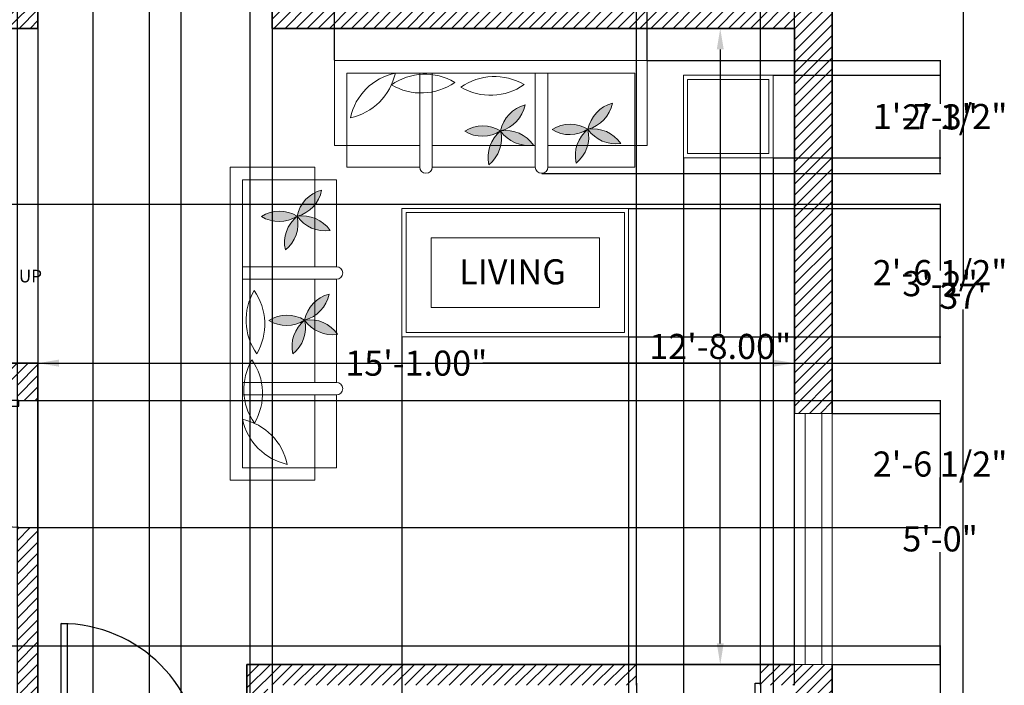
# Model space of a CAD drawing. Units: inches. Extents: x -302 to 383, y -29 to 550.
# Tile 3 of 4: x 147 to 383, y 149 to 308. Entities that reach past the tile are written whole.
import ezdxf

# ---------------------------------------------------------------- set-up
doc = ezdxf.new("R2010")
doc.units = ezdxf.units.IN
doc.header["$MEASUREMENT"] = 0
for name, color, linetype, lineweight in [('A-ANNO-DIMS', 3, 'Continuous', 18), ('A-ANNO-TEXT', 7, 'Continuous', 18), ('A-AREA-IDEN', 2, 'Continuous', 25), ('A-DOOR', 4, 'Continuous', 25), ('A-FURN', 1, 'Continuous', 18), ('A-FURN-PATT', 2, 'Continuous', 13), ('A-GLAZ', 2, 'Continuous', 18), ('A-WALL', 7, 'Continuous', 35), ('A-WALL-PATT', 252, 'Continuous', 13)]:
    doc.layers.add(name, color=color, linetype=linetype, lineweight=lineweight)
doc.styles.get("Standard").update_dxf_attribs({"font": 'arial.ttf'})
doc.dimstyles.get("Standard").update_dxf_attribs({"dimtxt": 6, "dimasz": 0.18, "dimexe": 0.18, "dimexo": 0.0625, "dimgap": 0.09, "dimtad": 0, "dimtih": 1, "dimtoh": 1, "dimzin": 0, "dimdsep": 46, "dimlunit": 3, "dimtxsty": 'Standard', "dimcen": 0.09, "dimadec": 0, "dimazin": 0, "dimtfac": 1, "dimtofl": 0, "dimtmove": 0, "dimatfit": 3, "dimfxl": 1, "dimtolj": 1, "dimtzin": 0, "dimarcsym": 0})

# ---------------------------------------------------------------- blocks, each defined once
blk = doc.blocks.new('*U2')
for p, q in [((0, 0), (0, -6)), ((40, 0), (40, -6))]:
    blk.add_line(p, q)
blk.add_lwpolyline([(0, 0), (0, 40), (1.75, 40), (1.75, 0)], close=True)
blk.add_arc((0, 0), 40, 0, 90)
blk = doc.blocks.new('*D13')
at = {"layer": 'A-ANNO-DIMS', "color": 0, "lineweight": -2, "transparency": 16777216}
for p, q in [((151.7, 226.34), (151.7, 226.45)), ((156.7, 226.27), (226.26, 226.27)), ((327.7, 226.27), (258.14, 226.27)), ((332.7, 226.34), (332.7, 226.45))]:
    blk.add_line(p, q, dxfattribs=at)
at = {"layer": 'A-ANNO-DIMS', "color": 0, "transparency": 16777216}
for points in [[(156.7, 227.11), (156.7, 225.44), (151.7, 226.27)], [(327.7, 227.11), (327.7, 225.44), (332.7, 226.27)]]:
    blk.add_solid(points, dxfattribs=at)
at = {"layer": 'Defpoints', "color": 0, "transparency": 16777216}
for p in [(151.7, 226.27), (332.7, 226.27), (332.7, 226.27)]:
    blk.add_point(p, dxfattribs=at)
at = {"layer": 'A-ANNO-DIMS', "color": 0, "transparency": 16777216, "insert": (242.2, 226.27), "char_height": 6, "attachment_point": 5}
blk.add_mtext('\\A1;15\'-1.00"', dxfattribs=at)
blk = doc.blocks.new('*D14')
at = {"layer": 'A-ANNO-DIMS', "color": 0, "lineweight": -2, "transparency": 16777216}
for p, q in [((332.63, 306.27), (314.73, 306.27)), ((314.91, 301.27), (314.91, 233.43)), ((314.91, 159.27), (314.91, 227.12)), ((332.63, 154.27), (314.73, 154.27))]:
    blk.add_line(p, q, dxfattribs=at)
at = {"layer": 'A-ANNO-DIMS', "color": 0, "transparency": 16777216}
for points in [[(314.08, 301.27), (315.74, 301.27), (314.91, 306.27)], [(314.08, 159.27), (315.74, 159.27), (314.91, 154.27)]]:
    blk.add_solid(points, dxfattribs=at)
at = {"layer": 'Defpoints', "color": 0, "transparency": 16777216}
for p in [(332.7, 306.27), (314.91, 154.27), (332.7, 154.27)]:
    blk.add_point(p, dxfattribs=at)
at = {"layer": 'A-ANNO-DIMS', "color": 0, "transparency": 16777216, "insert": (314.91, 230.27), "char_height": 6, "attachment_point": 5}
blk.add_mtext('\\A1;12\'-8.00"', dxfattribs=at)
blk = doc.blocks.new('*D22')
at = {"layer": 'A-ANNO-DIMS', "color": 0, "lineweight": -2, "transparency": 16777216}
for p, q in [((341.76, 464.27), (373.16, 464.27)), ((372.98, 459.27), (372.98, 245.43)), ((372.98, 25.27), (372.98, 239.12)), ((341.76, 20.27), (373.16, 20.27))]:
    blk.add_line(p, q, dxfattribs=at)
at = {"layer": 'A-ANNO-DIMS', "color": 0, "transparency": 16777216}
for points in [[(372.15, 459.27), (373.82, 459.27), (372.98, 464.27)], [(372.15, 25.27), (373.82, 25.27), (372.98, 20.27)]]:
    blk.add_solid(points, dxfattribs=at)
at = {"layer": 'Defpoints', "color": 0, "transparency": 16777216}
for p in [(341.7, 464.27), (341.7, 20.27), (372.98, 20.27)]:
    blk.add_point(p, dxfattribs=at)
at = {"layer": 'A-ANNO-DIMS', "color": 0, "transparency": 16777216, "insert": (372.98, 242.27), "char_height": 6, "attachment_point": 5}
blk.add_mtext("\\A1;37'", dxfattribs=at)
blk = doc.blocks.new('SOFA-LEAF-TRIO')
for points in [[(0, 0, 0.294318), (10.77, 10.69, 0.294318)], [(9.82, 7.86, 0.294318), (24.97, 8.46, 0.294318)], [(26.41, 7.31, 0.294318), (41.57, 7.92, 0.294318)]]:
    blk.add_lwpolyline(points, format="xyb", close=True)
blk = doc.blocks.new('SOFA-FLORAL-MOTIF-A')
h = blk.add_hatch(color=256)
h.dxf.hatch_style = 1
h.paths.add_polyline_path([(0, 8, 0.287656), (8.55, 8.07, 0.287656)])
h.paths.add_polyline_path([(14.4, 14.32, 0.287656), (8.55, 8.07, 0.287656)])
h.paths.add_polyline_path([(8.55, 8.07, 0.287656), (5.73, 0, 0.287656)])
h.paths.add_polyline_path([(8.55, 8.07, 0.287656), (16.41, 4.69, 0.287656)])
for centre, start, end in [((16.45, 6.53), 104.7854, 168.9781), ((6.5, 15.85), 284.7854, 348.9781), ((4.34, 1.22), 58.4247, 122.6174), ((4.21, 14.85), 238.4247, 302.6174), ((13.58, 1.79), 128.6278, 192.8205), ((0.7, 6.29), 308.6278, 12.8205), ((9.78, 0.12), 34.5823, 98.775), ((15.18, 12.64), 214.5823, 278.775)]:
    blk.add_arc(centre, 8.05, start, end)
blk = doc.blocks.new('SOFA-FLORAL-MOTIF-B')
h = blk.add_hatch(color=256)
h.dxf.hatch_style = 1
h.paths.add_polyline_path([(0, 8, 0.287656), (8.55, 8.07, 0.287656)])
h.paths.add_polyline_path([(14.4, 14.32, 0.287656), (8.55, 8.07, 0.287656)])
h.paths.add_polyline_path([(5.73, 0, 0.287656), (8.55, 8.07, 0.287656)])
h.paths.add_polyline_path([(16.41, 4.69, 0.287656), (8.55, 8.07, 0.287656)])
for centre, start, end in [((16.45, 6.53), 104.7854, 168.9781), ((6.5, 15.85), 284.7854, 348.9781), ((4.34, 1.22), 58.4247, 122.6174), ((4.21, 14.85), 238.4247, 302.6174), ((13.58, 1.79), 128.6278, 192.8205), ((0.7, 6.29), 308.6278, 12.8205), ((9.78, 0.12), 34.5823, 98.775), ((15.18, 12.64), 214.5823, 278.775)]:
    blk.add_arc(centre, 8.05, start, end)
blk = doc.blocks.new('*D33')
at = {"layer": 'A-ANNO-DIMS', "color": 0, "lineweight": -2, "transparency": 16777216}
for p, q in [((210.8, 127.61), (210.8, 125.91)), ((221.35, 127.61), (221.35, 125.91)), ((210.98, 126.09), (221.17, 126.09)), ((221.35, 126.09), (221.53, 126.09))]:
    blk.add_line(p, q, dxfattribs=at)
at = {"layer": 'A-ANNO-DIMS', "color": 0, "transparency": 16777216}
for points in [[(210.98, 126.12), (210.98, 126.06), (210.8, 126.09)], [(221.17, 126.12), (221.17, 126.06), (221.35, 126.09)]]:
    blk.add_solid(points, dxfattribs=at)
at = {"layer": 'Defpoints', "color": 0, "transparency": 16777216}
for p in [(210.8, 127.68), (221.35, 127.68), (221.35, 126.09)]:
    blk.add_point(p, dxfattribs=at)
at = {"layer": 'A-ANNO-DIMS', "color": 0, "transparency": 16777216, "insert": (276.32, 126.09), "char_height": 6, "attachment_point": 5}
blk.add_mtext('\\A1;TABLE LAMP 0\'-10 1/2" TYP.', dxfattribs=at)
blk = doc.blocks.new('*D45')
at = {"layer": 'A-ANNO-DIMS', "color": 0, "lineweight": -2, "transparency": 16777216}
for p, q in [((341.76, 214.27), (367.68, 214.27)), ((367.5, 214.09), (367.5, 187.43)), ((367.5, 154.45), (367.5, 181.12)), ((341.76, 154.27), (367.68, 154.27))]:
    blk.add_line(p, q, dxfattribs=at)
at = {"layer": 'A-ANNO-DIMS', "color": 0, "transparency": 16777216}
for points in [[(367.47, 214.09), (367.53, 214.09), (367.5, 214.27)], [(367.47, 154.45), (367.53, 154.45), (367.5, 154.27)]]:
    blk.add_solid(points, dxfattribs=at)
at = {"layer": 'Defpoints', "color": 0, "transparency": 16777216}
for p in [(341.7, 214.27), (367.5, 214.27), (341.7, 154.27)]:
    blk.add_point(p, dxfattribs=at)
at = {"layer": 'A-ANNO-DIMS', "color": 0, "transparency": 16777216, "insert": (367.5, 184.27), "char_height": 6, "attachment_point": 5}
blk.add_mtext('\\A1;5\'-0"', dxfattribs=at)
blk = doc.blocks.new('*D50')
at = {"layer": 'A-ANNO-DIMS', "color": 0, "lineweight": -2, "transparency": 16777216}
for p, q in [((178.34, 359.21), (178.34, -5.71)), ((202.4, 359.21), (202.4, -5.71)), ((178.52, -5.53), (182.25, -5.53)), ((202.22, -5.53), (198.48, -5.53))]:
    blk.add_line(p, q, dxfattribs=at)
at = {"layer": 'A-ANNO-DIMS', "color": 0, "transparency": 16777216}
for points in [[(178.52, -5.5), (178.52, -5.56), (178.34, -5.53)], [(202.22, -5.5), (202.22, -5.56), (202.4, -5.53)]]:
    blk.add_solid(points, dxfattribs=at)
at = {"layer": 'Defpoints', "color": 0, "transparency": 16777216}
for p in [(178.34, 359.27), (202.4, 359.27), (202.4, -5.53)]:
    blk.add_point(p, dxfattribs=at)
at = {"layer": 'A-ANNO-DIMS', "color": 0, "transparency": 16777216, "insert": (190.37, -5.53), "char_height": 6, "attachment_point": 5}
blk.add_mtext('\\A1;2\'-0"', dxfattribs=at)
blk = doc.blocks.new('*D51')
at = {"layer": 'A-ANNO-DIMS', "color": 0, "lineweight": -2, "transparency": 16777216}
for p, q in [((146.76, 217.32), (367.68, 217.32)), ((367.5, 217.14), (367.5, 205.35)), ((367.5, 187.18), (367.5, 198.97)), ((146.76, 187), (367.68, 187))]:
    blk.add_line(p, q, dxfattribs=at)
at = {"layer": 'A-ANNO-DIMS', "color": 0, "transparency": 16777216}
for points in [[(367.47, 217.14), (367.53, 217.14), (367.5, 217.32)], [(367.47, 187.18), (367.53, 187.18), (367.5, 187)]]:
    blk.add_solid(points, dxfattribs=at)
at = {"layer": 'Defpoints', "color": 0, "transparency": 16777216}
for p in [(146.7, 217.32), (367.5, 217.32), (146.7, 187)]:
    blk.add_point(p, dxfattribs=at)
at = {"layer": 'A-ANNO-DIMS', "color": 0, "transparency": 16777216, "insert": (367.5, 202.16), "char_height": 6, "attachment_point": 5}
blk.add_mtext('\\A1;2\'-6 1/2"', dxfattribs=at)
blk = doc.blocks.new('*D53')
at = {"layer": 'A-ANNO-DIMS', "color": 0, "lineweight": -2, "transparency": 16777216}
for p, q in [((294.85, 149.34), (294.85, 541.25)), ((295.03, 541.07), (324.38, 541.07)), ((324.56, 149.34), (324.56, 541.25)), ((324.56, 541.07), (324.74, 541.07))]:
    blk.add_line(p, q, dxfattribs=at)
at = {"layer": 'A-ANNO-DIMS', "color": 0, "transparency": 16777216}
for points in [[(295.03, 541.1), (295.03, 541.04), (294.85, 541.07)], [(324.38, 541.1), (324.38, 541.04), (324.56, 541.07)]]:
    blk.add_solid(points, dxfattribs=at)
at = {"layer": 'Defpoints', "color": 0, "transparency": 16777216}
for p in [(324.56, 541.07), (294.85, 149.27), (324.56, 149.27)]:
    blk.add_point(p, dxfattribs=at)
at = {"layer": 'A-ANNO-DIMS', "color": 0, "transparency": 16777216, "insert": (339.85, 541.07), "char_height": 6, "attachment_point": 5}
blk.add_mtext('\\A1;2\'-5 1/2"', dxfattribs=at)
blk = doc.blocks.new('*D56')
at = {"layer": 'A-ANNO-DIMS', "color": 0, "lineweight": -2, "transparency": 16777216}
for p, q in [((134.76, 264.27), (367.68, 264.27)), ((367.5, 264.09), (367.5, 248.43)), ((367.5, 226.45), (367.5, 242.12)), ((134.76, 226.27), (367.68, 226.27))]:
    blk.add_line(p, q, dxfattribs=at)
at = {"layer": 'A-ANNO-DIMS', "color": 0, "transparency": 16777216}
for points in [[(367.47, 264.09), (367.53, 264.09), (367.5, 264.27)], [(367.47, 226.45), (367.53, 226.45), (367.5, 226.27)]]:
    blk.add_solid(points, dxfattribs=at)
at = {"layer": 'Defpoints', "color": 0, "transparency": 16777216}
for p in [(134.7, 264.27), (367.5, 264.27), (134.7, 226.27)]:
    blk.add_point(p, dxfattribs=at)
at = {"layer": 'A-ANNO-DIMS', "color": 0, "transparency": 16777216, "insert": (367.5, 245.27), "char_height": 6, "attachment_point": 5}
blk.add_mtext('\\A1;3\'-2"', dxfattribs=at)
blk = doc.blocks.new('*D58')
at = {"layer": 'A-ANNO-DIMS', "color": 0, "lineweight": -2, "transparency": 16777216}
for p, q in [((50.76, 158.73), (367.68, 158.73)), ((367.5, 158.55), (367.5, 109.19)), ((367.5, 53.45), (367.5, 102.81)), ((50.76, 53.27), (367.68, 53.27))]:
    blk.add_line(p, q, dxfattribs=at)
at = {"layer": 'A-ANNO-DIMS', "color": 0, "transparency": 16777216}
for points in [[(367.47, 158.55), (367.53, 158.55), (367.5, 158.73)], [(367.47, 53.45), (367.53, 53.45), (367.5, 53.27)]]:
    blk.add_solid(points, dxfattribs=at)
at = {"layer": 'Defpoints', "color": 0, "transparency": 16777216}
for p in [(50.7, 158.73), (367.5, 158.73), (50.7, 53.27)]:
    blk.add_point(p, dxfattribs=at)
at = {"layer": 'A-ANNO-DIMS', "color": 0, "transparency": 16777216, "insert": (367.5, 106), "char_height": 6, "attachment_point": 5}
blk.add_mtext('\\A1;8\'-9 1/2"', dxfattribs=at)
blk = doc.blocks.new('*D60')
at = {"layer": 'A-ANNO-DIMS', "color": 0, "lineweight": -2, "transparency": 16777216}
for p, q in [((164.84, 447.21), (164.84, -5.71)), ((185.84, 447.21), (185.84, -5.71)), ((165.02, -5.53), (167.56, -5.53)), ((185.66, -5.53), (183.12, -5.53))]:
    blk.add_line(p, q, dxfattribs=at)
at = {"layer": 'A-ANNO-DIMS', "color": 0, "transparency": 16777216}
for points in [[(165.02, -5.5), (165.02, -5.56), (164.84, -5.53)], [(185.66, -5.5), (185.66, -5.56), (185.84, -5.53)]]:
    blk.add_solid(points, dxfattribs=at)
at = {"layer": 'Defpoints', "color": 0, "transparency": 16777216}
for p in [(164.84, 447.27), (185.84, 447.27), (185.84, -5.53)]:
    blk.add_point(p, dxfattribs=at)
at = {"layer": 'A-ANNO-DIMS', "color": 0, "transparency": 16777216, "insert": (175.34, -5.53), "char_height": 6, "attachment_point": 5}
blk.add_mtext('\\A1;1\'-9"', dxfattribs=at)
blk = doc.blocks.new('*D62')
at = {"layer": 'A-ANNO-DIMS', "color": 0, "lineweight": -2, "transparency": 16777216}
for p, q in [((222.62, 298.67), (222.62, 541.25)), ((222.8, 541.07), (251.95, 541.07)), ((297.27, 541.07), (268.11, 541.07)), ((297.45, 298.67), (297.45, 541.25))]:
    blk.add_line(p, q, dxfattribs=at)
at = {"layer": 'A-ANNO-DIMS', "color": 0, "transparency": 16777216}
for points in [[(222.8, 541.1), (222.8, 541.04), (222.62, 541.07)], [(297.27, 541.1), (297.27, 541.04), (297.45, 541.07)]]:
    blk.add_solid(points, dxfattribs=at)
at = {"layer": 'Defpoints', "color": 0, "transparency": 16777216}
for p in [(297.45, 541.07), (222.62, 298.61), (297.45, 298.61)]:
    blk.add_point(p, dxfattribs=at)
at = {"layer": 'A-ANNO-DIMS', "color": 0, "transparency": 16777216, "insert": (260.03, 541.07), "char_height": 6, "attachment_point": 5}
blk.add_mtext('\\A1;6\'-3"', dxfattribs=at)
blk = doc.blocks.new('*D63')
at = {"layer": 'A-ANNO-DIMS', "color": 0, "lineweight": -2, "transparency": 16777216}
for p, q in [((297.51, 298.61), (367.68, 298.61)), ((367.5, 298.43), (367.5, 288.28)), ((367.5, 271.82), (367.5, 281.97)), ((272.23, 271.64), (367.68, 271.64))]:
    blk.add_line(p, q, dxfattribs=at)
at = {"layer": 'A-ANNO-DIMS', "color": 0, "transparency": 16777216}
for points in [[(367.47, 298.43), (367.53, 298.43), (367.5, 298.61)], [(367.47, 271.82), (367.53, 271.82), (367.5, 271.64)]]:
    blk.add_solid(points, dxfattribs=at)
at = {"layer": 'Defpoints', "color": 0, "transparency": 16777216}
for p in [(297.45, 298.61), (272.17, 271.64), (367.5, 271.64)]:
    blk.add_point(p, dxfattribs=at)
at = {"layer": 'A-ANNO-DIMS', "color": 0, "transparency": 16777216, "insert": (367.5, 285.13), "char_height": 6, "attachment_point": 5}
blk.add_mtext('\\A1;2\'-3"', dxfattribs=at)
blk = doc.blocks.new('*D64')
at = {"layer": 'A-ANNO-DIMS', "color": 0, "lineweight": -2, "transparency": 16777216}
for p, q in [((238.76, 232.51), (238.76, -5.71)), ((292.99, 232.51), (292.99, -5.71)), ((238.94, -5.53), (257.69, -5.53)), ((292.81, -5.53), (274.06, -5.53))]:
    blk.add_line(p, q, dxfattribs=at)
at = {"layer": 'A-ANNO-DIMS', "color": 0, "transparency": 16777216}
for points in [[(238.94, -5.5), (238.94, -5.56), (238.76, -5.53)], [(292.81, -5.5), (292.81, -5.56), (292.99, -5.53)]]:
    blk.add_solid(points, dxfattribs=at)
at = {"layer": 'Defpoints', "color": 0, "transparency": 16777216}
for p in [(238.76, 232.57), (292.99, 232.57), (292.99, -5.53)]:
    blk.add_point(p, dxfattribs=at)
at = {"layer": 'A-ANNO-DIMS', "color": 0, "transparency": 16777216, "insert": (265.88, -5.53), "char_height": 6, "attachment_point": 5}
blk.add_mtext('\\A1;4\'-6"', dxfattribs=at)
blk = doc.blocks.new('*D65')
at = {"layer": 'A-ANNO-DIMS', "color": 0, "lineweight": -2, "transparency": 16777216}
for p, q in [((293.06, 263.25), (367.68, 263.25)), ((367.5, 263.07), (367.5, 251.1)), ((367.5, 232.75), (367.5, 244.72)), ((293.06, 232.57), (367.68, 232.57))]:
    blk.add_line(p, q, dxfattribs=at)
at = {"layer": 'A-ANNO-DIMS', "color": 0, "transparency": 16777216}
for points in [[(367.47, 263.07), (367.53, 263.07), (367.5, 263.25)], [(367.47, 232.75), (367.53, 232.75), (367.5, 232.57)]]:
    blk.add_solid(points, dxfattribs=at)
at = {"layer": 'Defpoints', "color": 0, "transparency": 16777216}
for p in [(292.99, 263.25), (367.5, 263.25), (292.99, 232.57)]:
    blk.add_point(p, dxfattribs=at)
at = {"layer": 'A-ANNO-DIMS', "color": 0, "transparency": 16777216, "insert": (367.5, 247.91), "char_height": 6, "attachment_point": 5}
blk.add_mtext('\\A1;2\'-6 1/2"', dxfattribs=at)
blk = doc.blocks.new('*D71')
at = {"layer": 'A-ANNO-DIMS', "color": 0, "lineweight": -2, "transparency": 16777216}
for p, q in [((146.7, 358.81), (146.7, -5.71)), ((151.7, 354.21), (151.7, -5.71)), ((146.88, -5.53), (151.52, -5.53)), ((151.7, -5.53), (151.88, -5.53))]:
    blk.add_line(p, q, dxfattribs=at)
at = {"layer": 'A-ANNO-DIMS', "color": 0, "transparency": 16777216}
for points in [[(146.88, -5.5), (146.88, -5.56), (146.7, -5.53)], [(151.52, -5.5), (151.52, -5.56), (151.7, -5.53)]]:
    blk.add_solid(points, dxfattribs=at)
at = {"layer": 'Defpoints', "color": 0, "transparency": 16777216}
for p in [(146.7, 358.87), (151.7, 354.27), (151.7, -5.53)]:
    blk.add_point(p, dxfattribs=at)
at = {"layer": 'A-ANNO-DIMS', "color": 0, "transparency": 16777216, "insert": (159.94, -5.53), "char_height": 6, "attachment_point": 5}
blk.add_mtext('\\A1;0\'-5"', dxfattribs=at)
blk = doc.blocks.new('*D72')
at = {"layer": 'A-ANNO-DIMS', "color": 0, "lineweight": -2, "transparency": 16777216}
for p, q in [((202.4, 354.21), (202.4, -5.71)), ((207.7, 354.21), (207.7, -5.71)), ((202.58, -5.53), (207.52, -5.53)), ((207.7, -5.53), (207.88, -5.53))]:
    blk.add_line(p, q, dxfattribs=at)
at = {"layer": 'A-ANNO-DIMS', "color": 0, "transparency": 16777216}
for points in [[(202.58, -5.5), (202.58, -5.56), (202.4, -5.53)], [(207.52, -5.5), (207.52, -5.56), (207.7, -5.53)]]:
    blk.add_solid(points, dxfattribs=at)
at = {"layer": 'Defpoints', "color": 0, "transparency": 16777216}
for p in [(202.4, 354.27), (207.7, 354.27), (207.7, -5.53)]:
    blk.add_point(p, dxfattribs=at)
at = {"layer": 'A-ANNO-DIMS', "color": 0, "transparency": 16777216, "insert": (222.93, -5.53), "char_height": 6, "attachment_point": 5}
blk.add_mtext('\\A1;0\'-5 1/2"', dxfattribs=at)
blk = doc.blocks.new('*D74')
at = {"layer": 'A-ANNO-DIMS', "color": 0, "lineweight": -2, "transparency": 16777216}
for p, q in [((324.56, 149.34), (324.56, 541.25)), ((324.74, 541.07), (332.52, 541.07)), ((332.7, 149.34), (332.7, 541.25)), ((332.7, 541.07), (332.88, 541.07))]:
    blk.add_line(p, q, dxfattribs=at)
at = {"layer": 'A-ANNO-DIMS', "color": 0, "transparency": 16777216}
for points in [[(324.74, 541.1), (324.74, 541.04), (324.56, 541.07)], [(332.52, 541.1), (332.52, 541.04), (332.7, 541.07)]]:
    blk.add_solid(points, dxfattribs=at)
at = {"layer": 'Defpoints', "color": 0, "transparency": 16777216}
for p in [(332.7, 541.07), (324.56, 149.27), (332.7, 149.27)]:
    blk.add_point(p, dxfattribs=at)
at = {"layer": 'A-ANNO-DIMS', "color": 0, "transparency": 16777216, "insert": (340.94, 541.07), "char_height": 6, "attachment_point": 5}
blk.add_mtext('\\A1;0\'-8"', dxfattribs=at)
blk = doc.blocks.new('*D77')
at = {"layer": 'A-ANNO-DIMS', "color": 0, "lineweight": -2, "transparency": 16777216}
for p, q in [((306.08, 275.31), (306.08, -5.71)), ((327.55, 275.31), (327.55, -5.71)), ((306.26, -5.53), (327.37, -5.53)), ((327.55, -5.53), (327.73, -5.53))]:
    blk.add_line(p, q, dxfattribs=at)
at = {"layer": 'A-ANNO-DIMS', "color": 0, "transparency": 16777216}
for points in [[(306.26, -5.5), (306.26, -5.56), (306.08, -5.53)], [(327.37, -5.5), (327.37, -5.56), (327.55, -5.53)]]:
    blk.add_solid(points, dxfattribs=at)
at = {"layer": 'Defpoints', "color": 0, "transparency": 16777216}
for p in [(306.08, 275.38), (327.55, 275.38), (327.55, -5.53)]:
    blk.add_point(p, dxfattribs=at)
at = {"layer": 'A-ANNO-DIMS', "color": 0, "transparency": 16777216, "insert": (342.5, -5.53), "char_height": 6, "attachment_point": 5}
blk.add_mtext('\\A1;1\'-9 1/2"', dxfattribs=at)
blk = doc.blocks.new('*D78')
at = {"layer": 'A-ANNO-DIMS', "color": 0, "lineweight": -2, "transparency": 16777216}
for p, q in [((327.61, 295.09), (367.68, 295.09)), ((367.5, 294.91), (367.5, 288.43)), ((367.5, 275.56), (367.5, 282.04)), ((327.61, 275.38), (367.68, 275.38))]:
    blk.add_line(p, q, dxfattribs=at)
at = {"layer": 'A-ANNO-DIMS', "color": 0, "transparency": 16777216}
for points in [[(367.47, 294.91), (367.53, 294.91), (367.5, 295.09)], [(367.47, 275.56), (367.53, 275.56), (367.5, 275.38)]]:
    blk.add_solid(points, dxfattribs=at)
at = {"layer": 'Defpoints', "color": 0, "transparency": 16777216}
for p in [(327.55, 295.09), (367.5, 295.09), (327.55, 275.38)]:
    blk.add_point(p, dxfattribs=at)
at = {"layer": 'A-ANNO-DIMS', "color": 0, "transparency": 16777216, "insert": (367.5, 285.23), "char_height": 6, "attachment_point": 5}
blk.add_mtext('\\A1;1\'-7 1/2"', dxfattribs=at)

msp = doc.modelspace()

# ---------------------------------------------------------------- hatches: boundary and pattern name
at = {"layer": 'A-WALL-PATT'}
h = msp.add_hatch(dxfattribs=at)
h.set_pattern_fill('ANSI31', color=256, scale=15)
h.paths.add_polyline_path([(201.697, 29.273), (187.202, 29.273), (187.202, 20.273), (251.158, 20.273), (251.158, 29.273), (206.697, 29.273), (206.697, 149.273), (294.846, 149.273, -0.0045588), (294.841, 149.815), (294.841, 154.273), (201.697, 154.273), (201.697, 130.273), (190.923, 130.273), (190.923, 125.273), (201.697, 125.273)])
h.paths.add_polyline_path([(341.697, 154.273), (332.697, 154.273), (324.561, 154.273), (324.561, 149.815), (324.561, 149.273), (332.697, 149.273), (332.697, 29.273), (299.158, 29.273), (299.158, 20.273), (341.697, 20.273)])
h.paths.add_polyline_path([(75.47, 20.273), (75.47, 29.273), (26.697, 29.273), (26.697, 89.142), (17.697, 89.142), (17.697, 20.273)])
h.paths.add_polyline_path([(26.697, 221.273), (146.697, 221.273), (146.697, 217.323), (147.147, 217.323), (151.697, 217.323), (151.697, 226.273), (26.697, 226.273), (26.697, 248.984), (17.697, 248.984), (17.697, 137.142), (26.697, 137.142)])
h.paths.add_polyline_path([(17.697, 284.934), (26.697, 284.934), (26.697, 306.273), (151.697, 306.273), (151.697, 317.511), (147.338, 317.511), (146.697, 317.511), (146.697, 311.273), (26.697, 311.273), (26.697, 377.22), (17.697, 377.22)])
h.paths.add_polyline_path([(341.697, 376.674), (332.697, 376.674), (332.697, 311.273), (212.697, 311.273), (212.697, 317.511), (212.055, 317.511), (207.697, 317.511), (207.697, 306.273), (332.697, 306.273), (332.697, 214.273), (341.697, 214.273)])
h.paths.add_polyline_path([(207.697, 455.273), (207.697, 359.273), (202.395, 359.273), (202.395, 357.888), (202.395, 354.273), (207.697, 354.273), (207.697, 346.57), (212.055, 346.57, -0.0055163), (212.697, 346.563), (212.697, 455.273), (332.697, 455.273), (332.697, 424.674), (341.697, 424.674), (341.697, 464.273), (188.075, 464.273), (188.075, 455.273)])
h.paths.add_polyline_path([(17.697, 464.273), (17.697, 425.22), (26.697, 425.22), (26.697, 455.273), (146.697, 455.273), (146.697, 346.563, -0.0055163), (147.338, 346.57), (151.697, 346.57), (151.697, 354.273), (178.3, 354.273), (178.3, 357.888, -0.0143868), (178.34, 359.273), (151.697, 359.273), (151.697, 455.273), (162.634, 455.273), (162.634, 464.273)])
h = msp.add_hatch(dxfattribs=at)
h.set_pattern_fill('ANSI31', color=256, scale=15)
h.paths.add_polyline_path([(151.697, 186.995), (147.147, 186.995, -0.0037161), (146.697, 186.998), (146.697, 29.273), (123.47, 29.273), (123.47, 20.273), (162.437, 20.273), (162.437, 29.273), (151.697, 29.273), (151.697, 125.273), (157.23, 125.273), (157.23, 130.273), (151.697, 130.273)])

# ---------------------------------------------------------------- linework, layer by layer
at = {"layer": 'A-FURN'}
for p, q in [((243.019, 295.611), (243.019, 273.144)), ((246.019, 295.611), (246.019, 273.144)), ((270.669, 295.611), (270.669, 273.144)), ((273.669, 295.611), (273.669, 273.144))]:
    msp.add_line(p, q, dxfattribs=at)
for points in [[(222.615, 278.325), (222.615, 298.611), (297.448, 298.611), (297.448, 278.325), (273.669, 278.325)], [(243.019, 273.144), (225.615, 273.144), (225.615, 295.611), (294.448, 295.611), (294.448, 273.144), (273.669, 273.144)], [(243.019, 278.325), (222.615, 278.325)], [(270.669, 278.325), (246.019, 278.325)], [(217.945, 218.681), (217.945, 198.277), (197.659, 198.277), (197.659, 273.11), (217.945, 273.11), (217.945, 249.331)], [(270.669, 273.144), (246.019, 273.144)], [(223.126, 218.681), (223.126, 201.277), (200.659, 201.277), (200.659, 270.11), (223.126, 270.11), (223.126, 249.331)], [(217.945, 246.331), (217.945, 221.681)], [(223.126, 246.331), (223.126, 221.681)]]:
    msp.add_lwpolyline(points, dxfattribs=at)
for points in [[(306.081, 295.091), (327.545, 295.091), (327.545, 275.376), (306.081, 275.376)], [(307.081, 294.091), (326.545, 294.091), (326.545, 276.376), (307.081, 276.376)], [(238.759, 263.252), (292.993, 263.252), (292.993, 232.573), (238.759, 232.573)], [(239.759, 262.252), (291.993, 262.252), (291.993, 233.573), (239.759, 233.573)], [(245.759, 256.252), (285.993, 256.252), (285.993, 239.573), (245.759, 239.573)]]:
    msp.add_lwpolyline(points, close=True, dxfattribs=at)
for points in [[(200.659, 246.331), (223.126, 246.331, 1), (223.126, 249.331), (200.659, 249.331)], [(200.659, 218.681), (223.126, 218.681, 1), (223.126, 221.681), (200.659, 221.681)]]:
    msp.add_lwpolyline(points, format="xyb", dxfattribs=at)
for centre in [(244.519, 273.144), (272.169, 273.144)]:
    msp.add_arc(centre, 1.5, 180, 0, dxfattribs=at)
at = {"layer": 'A-GLAZ'}
msp.add_lwpolyline([(332.697, 214.273), (341.697, 214.273), (341.697, 154.273), (332.697, 154.273)], close=True, dxfattribs=at)
for points in [[(335.197, 154.273), (335.197, 214.273)], [(339.197, 154.273), (339.197, 214.273)]]:
    msp.add_lwpolyline(points, dxfattribs=at)
at = {"layer": 'A-WALL'}
for points in [[(341.697, 214.273), (341.697, 376.674)], [(151.697, 354.273), (151.697, 306.273)], [(207.697, 306.273), (207.697, 354.273)], [(151.697, 306.273), (26.697, 306.273)], [(332.697, 306.273), (207.697, 306.273)], [(332.697, 214.273), (332.697, 306.273)], [(26.697, 226.273), (151.697, 226.273)], [(151.697, 226.273), (151.697, 130.273)], [(201.697, 154.273), (332.697, 154.273)], [(201.697, 130.273), (201.697, 154.273)], [(299.158, 20.273), (341.697, 20.273), (341.697, 154.273)]]:
    msp.add_lwpolyline(points, dxfattribs=at)

# ---------------------------------------------------------------- block references
at = {"layer": 'A-DOOR'}
for p, xscale, yscale, zscale, rotation in [((147.147, 217.323), -0.7582020296560713, 0.7582020296560713, 0.7582020296560713, 90), ((324.561, 149.815), 0.7430126011318324, 0.7430126011318324, 0.7430126011318324, 180)]:
    msp.add_blockref('*U2', p, dxfattribs=dict(at, xscale=xscale, yscale=yscale, zscale=zscale, rotation=rotation))
at = {"layer": 'A-DOOR', "xscale": 0.8423175493774062, "yscale": 0.8423175493774062, "zscale": 0.8423175493774062}
msp.add_blockref('*U2', (157.23, 130.327), dxfattribs=at)
at = {"layer": 'A-FURN-PATT'}
for name, p in [('SOFA-LEAF-TRIO', (226.425, 284.926)), ('SOFA-FLORAL-MOTIF-A', (253.828, 273.704)), ('SOFA-FLORAL-MOTIF-A', (274.703, 274.097)), ('SOFA-FLORAL-MOTIF-B', (205.158, 253.323)), ('SOFA-FLORAL-MOTIF-B', (206.937, 228.473))]:
    msp.add_blockref(name, p, dxfattribs=at)
at = {"layer": 'A-FURN-PATT', "rotation": 90.00000000000088}
msp.add_blockref('SOFA-LEAF-TRIO', (211.345, 202.087), dxfattribs=at)

# ---------------------------------------------------------------- texts
at = {"layer": 'A-ANNO-TEXT', "insert": (147.134, 248.582), "char_height": 3, "attachment_point": 1}
msp.add_mtext_dynamic_manual_height_columns('UP', width=22.0138, gutter_width=1, heights=[0], dxfattribs=at)
at = {"layer": 'A-AREA-IDEN', "insert": (252.455, 251.102), "char_height": 6, "attachment_point": 1}
msp.add_mtext_dynamic_manual_height_columns('{LIVING}', width=101.54109, gutter_width=1, heights=[0], dxfattribs=at)

# ---------------------------------------------------------------- dimensions: what is measured, and where the dimension line sits
at = {"layer": 'A-ANNO-DIMS'}
for base, p1, p2, override, picture, middle in [((324.561, 541.073), (294.846, 149.273), (324.561, 149.273), {"dimdec": 1, "dimlfac": 1, "dimrnd": 0, "dimzin": 1, "dimdsep": 46, "dimlunit": 4, "dimfrac": 2}, '*D53', (339.848, 541.073)), ((297.448, 541.073), (222.615, 298.611), (297.448, 298.611), {"dimdec": 1, "dimlfac": 1, "dimrnd": 0, "dimzin": 1, "dimdsep": 46, "dimlunit": 4, "dimfrac": 2}, '*D62', (260.032, 541.073)), ((332.697, 541.073), (324.561, 149.273), (332.697, 149.273), {"dimdec": 1, "dimlfac": 1, "dimrnd": 0, "dimzin": 1, "dimdsep": 46, "dimlunit": 4, "dimfrac": 2}, '*D74', (340.941, 541.073)), ((185.841, -5.527), (164.841, 447.273), (185.841, 447.273), {"dimdec": 1, "dimlfac": 1, "dimrnd": 0, "dimzin": 1, "dimdsep": 46, "dimlunit": 4, "dimfrac": 2}, '*D60', (175.341, -5.527)), ((151.697, -5.527), (146.697, 358.869), (151.697, 354.273), {"dimdec": 1, "dimlfac": 1, "dimrnd": 0, "dimzin": 1, "dimdsep": 46, "dimlunit": 4, "dimfrac": 2}, '*D71', (159.941, -5.527)), ((202.395, -5.527), (178.34, 359.273), (202.395, 359.273), {"dimdec": 1, "dimlfac": 1, "dimrnd": 0, "dimzin": 1, "dimdsep": 46, "dimlunit": 4, "dimfrac": 2}, '*D50', (190.367, -5.527)), ((207.697, -5.527), (202.395, 354.273), (207.697, 354.273), {"dimdec": 1, "dimlfac": 1, "dimrnd": 0, "dimzin": 1, "dimdsep": 46, "dimlunit": 4, "dimfrac": 2}, '*D72', (222.932, -5.527)), ((327.545, -5.527), (306.081, 275.376), (327.545, 275.376), {"dimdec": 1, "dimlfac": 1, "dimrnd": 0, "dimzin": 1, "dimdsep": 46, "dimlunit": 4, "dimfrac": 2}, '*D77', (342.498, -5.527)), ((292.993, -5.527), (238.759, 232.573), (292.993, 232.573), {"dimdec": 1, "dimlfac": 1, "dimrnd": 0, "dimzin": 1, "dimdsep": 46, "dimlunit": 4, "dimfrac": 2}, '*D64', (265.876, -5.527)), ((332.697, 226.273), (151.697, 226.273), (332.697, 226.273), {"dimasz": 5, "dimclrd": 0, "dimclre": 0, "dimclrt": 0}, '*D13', (242.197, 226.273))]:
    dim = msp.add_linear_dim(base=base, p1=p1, p2=p2, dimstyle='Standard', override=override, dxfattribs=at)
    dim.commit()
    dim.dimension.update_dxf_attribs({"geometry": picture, "text_midpoint": middle})
for base, p1, p2, override, picture, middle in [((372.983, 20.273), (341.697, 464.273), (341.697, 20.273), {"dimasz": 5, "dimclrd": 0, "dimclre": 0, "dimclrt": 0}, '*D22', (372.983, 242.273)), ((314.911, 154.273), (332.697, 306.273), (332.697, 154.273), {"dimasz": 5, "dimclrd": 0, "dimclre": 0, "dimclrt": 0}, '*D14', (314.911, 230.273)), ((367.497, 271.644), (297.448, 298.611), (272.169, 271.644), {"dimdec": 1, "dimlfac": 1, "dimrnd": 0, "dimzin": 1, "dimdsep": 46, "dimlunit": 4, "dimfrac": 2}, '*D63', (367.497, 285.128)), ((367.497, 295.091), (327.545, 275.376), (327.545, 295.091), {"dimdec": 1, "dimlfac": 1, "dimrnd": 0, "dimzin": 1, "dimdsep": 46, "dimlunit": 4, "dimfrac": 2}, '*D78', (367.497, 285.233)), ((367.497, 264.273), (134.697, 226.273), (134.697, 264.273), {"dimdec": 1, "dimlfac": 1, "dimrnd": 0, "dimzin": 1, "dimdsep": 46, "dimlunit": 4, "dimfrac": 2}, '*D56', (367.497, 245.273)), ((367.497, 263.252), (292.993, 232.573), (292.993, 263.252), {"dimdec": 1, "dimlfac": 1, "dimrnd": 0, "dimzin": 1, "dimdsep": 46, "dimlunit": 4, "dimfrac": 2}, '*D65', (367.497, 247.912)), ((367.497, 217.323), (146.697, 186.998), (146.697, 217.323), {"dimdec": 1, "dimlfac": 1, "dimrnd": 0, "dimzin": 1, "dimdsep": 46, "dimlunit": 4, "dimfrac": 2}, '*D51', (367.497, 202.16)), ((367.497, 214.273), (341.697, 154.273), (341.697, 214.273), {"dimdec": 1, "dimlfac": 1, "dimrnd": 0, "dimzin": 1, "dimdsep": 46, "dimlunit": 4, "dimfrac": 2}, '*D45', (367.497, 184.273)), ((367.497, 158.726), (50.697, 53.273), (50.697, 158.726), {"dimdec": 1, "dimlfac": 1, "dimrnd": 0, "dimzin": 1, "dimdsep": 46, "dimlunit": 4, "dimfrac": 2}, '*D58', (367.497, 106))]:
    dim = msp.add_linear_dim(base=base, p1=p1, p2=p2, angle=90, dimstyle='Standard', override=override, dxfattribs=at)
    dim.commit()
    dim.dimension.update_dxf_attribs({"geometry": picture, "text_midpoint": middle})
dim = msp.add_linear_dim(base=(221.35, 126.093), p1=(210.802, 127.675), p2=(221.35, 127.675), text='TABLE LAMP <> TYP.', dimstyle='Standard', override={"dimdec": 1, "dimlfac": 1, "dimrnd": 0, "dimzin": 1, "dimdsep": 46, "dimlunit": 4, "dimfrac": 2}, dxfattribs=at)
dim.commit()
dim.dimension.update_dxf_attribs({"geometry": '*D33', "text_midpoint": (276.322, 126.093)})

doc.saveas('drawing.dxf')
